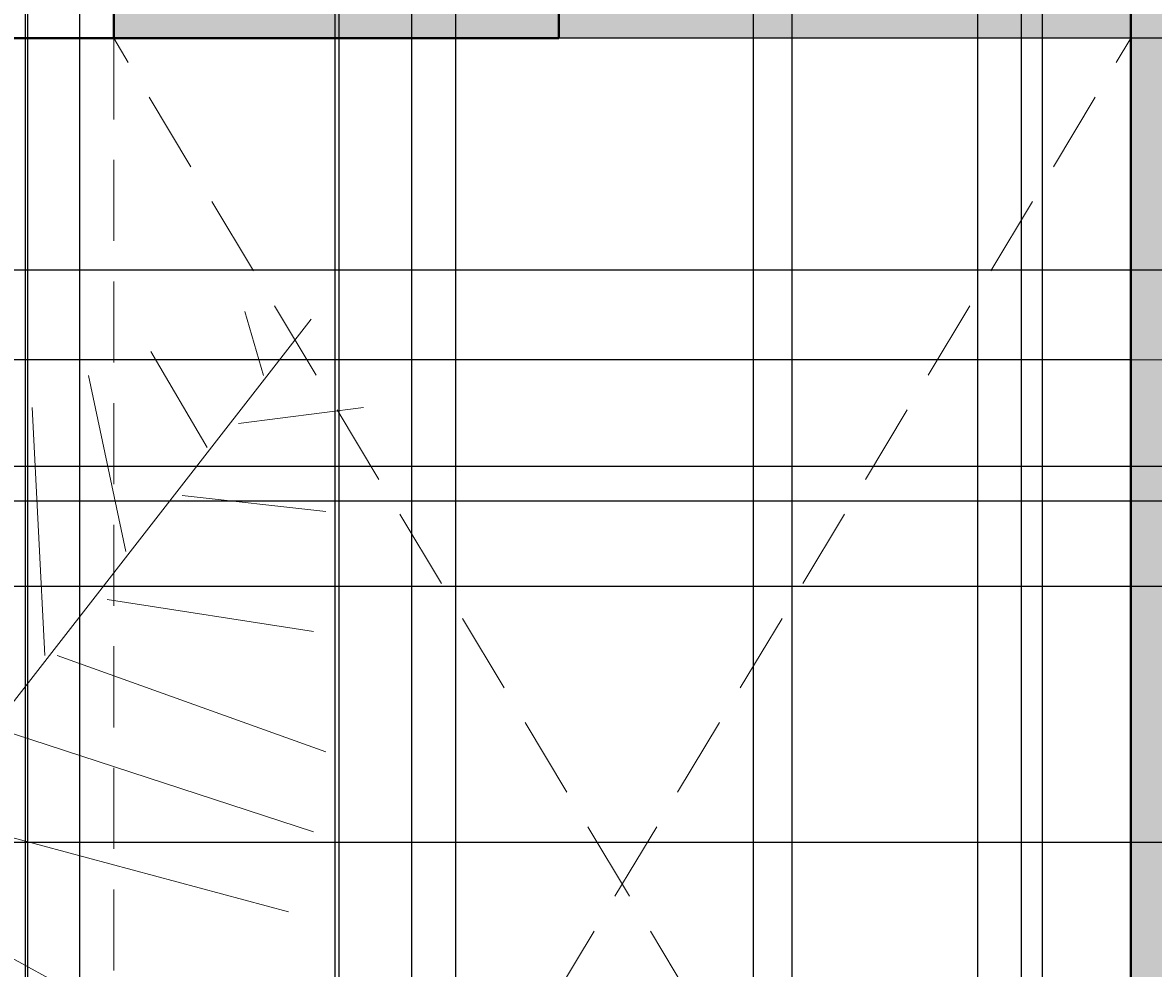
# Model space of a CAD drawing. Units: inches. Extents: x 818 to 1898, y 976 to 2364.
# Tile 65 of 96: x 1173 to 1260, y 1972 to 2045. Entities that reach past the tile are written whole.
import ezdxf

# ---------------------------------------------------------------- set-up
doc = ezdxf.new("R2010")
doc.units = ezdxf.units.IN
doc.header["$LTSCALE"] = 5
doc.header["$MEASUREMENT"] = 0
doc.linetypes.add('HIDDEN', pattern=[0.375, 0.25, -0.125])
for name, color, linetype, lineweight in [('A-ANNO-DIMS', 2, 'Continuous', 18), ('A-FLOR-OVHD', 8, 'HIDDEN', 13), ('A-GLAZ', 4, 'Continuous', 18), ('A-WALL', 7, 'Continuous', 40), ('A-WALL-HIDN', 7, 'HIDDEN', 18)]:
    doc.layers.add(name, color=color, linetype=linetype, lineweight=lineweight)
for name, color, linetype, lineweight, true_color in [('A-GLAZ-PATT', 141, 'Continuous', 9, 0xadddf7), ('A-WALL-PATT', 251, 'Continuous', 13, 0x636466), ('L-PLNT', 116, 'Continuous', 13, 0x136734)]:
    doc.layers.add(name, color=color, linetype=linetype, lineweight=lineweight, true_color=true_color)
doc.styles.get("Standard").update_dxf_attribs({"font": 'arial.ttf'})
doc.dimstyles.get("Standard").update_dxf_attribs({"dimtxt": 0.18, "dimasz": 0.18, "dimexe": 0.18, "dimexo": 0.0625, "dimgap": 0.09, "dimtad": 0, "dimtih": 1, "dimtoh": 1, "dimdec": 4, "dimzin": 0, "dimdsep": 46, "dimtxsty": 'Standard', "dimcen": 0.09, "dimadec": 0, "dimazin": 0, "dimtfac": 1, "dimtdec": 4, "dimtofl": 0, "dimtmove": 0, "dimatfit": 3, "dimfxl": 1, "dimtolj": 1, "dimtzin": 0, "dimarcsym": 0})

# ---------------------------------------------------------------- blocks, each defined once
blk = doc.blocks.new('PALM-DECK')
for p, q in [((132.87, 118.216), (134.313, 113.279)), ((110.075, 81.729), (137.983, 117.61)), ((125.649, 115.13), (129.981, 107.724)), ((120.834, 113.279), (123.723, 99.701)), ((116.502, 110.81), (117.465, 91.677)), ((132.389, 109.575), (142.017, 110.81)), ((128.056, 104.022), (139.128, 102.787)), ((122.279, 95.998), (138.165, 93.53)), ((118.427, 91.677), (139.128, 84.271)), ((113.613, 86.124), (138.165, 78.1)), ((106.393, 79.952), (136.239, 71.928)), ((98.208, 77.483), (120.834, 65.14))]:
    blk.add_line(p, q)
blk = doc.blocks.new('*D59')
at = {"layer": 'A-ANNO-DIMS', "color": 0, "lineweight": -2, "ltscale": 5, "transparency": 16777216}
for p, q in [((1251.643, 2300.393), (818.026, 2300.393)), ((818.206, 2300.213), (818.206, 1669.95)), ((818.206, 1039.323), (818.206, 1669.586)), ((896.051, 1039.143), (818.026, 1039.143))]:
    blk.add_line(p, q, dxfattribs=at)
at = {"layer": 'A-ANNO-DIMS', "color": 0, "ltscale": 5, "transparency": 16777216}
for points in [[(818.176, 2300.213), (818.236, 2300.213), (818.206, 2300.393)], [(818.176, 1039.323), (818.236, 1039.323), (818.206, 1039.143)]]:
    blk.add_solid(points, dxfattribs=at)
at = {"layer": 'Defpoints', "color": 0, "ltscale": 5, "transparency": 16777216}
for p in [(818.206, 2300.393), (1251.706, 2300.393), (896.114, 1039.143)]:
    blk.add_point(p, dxfattribs=at)
at = {"layer": 'A-ANNO-DIMS', "color": 0, "ltscale": 5, "transparency": 16777216, "insert": (818.206, 1669.768), "char_height": 0.18, "attachment_point": 5}
blk.add_mtext('\\A1;1261.2', dxfattribs=at)
blk = doc.blocks.new('*D61')
at = {"layer": 'A-ANNO-DIMS', "color": 0, "lineweight": -2, "ltscale": 5, "transparency": 16777216}
for p, q in [((1071.725, 1203.027), (1071.725, 2363.873)), ((1071.905, 2363.693), (1250.936, 2363.693)), ((1430.545, 2363.693), (1251.514, 2363.693)), ((1430.725, 1203.027), (1430.725, 2363.873))]:
    blk.add_line(p, q, dxfattribs=at)
at = {"layer": 'A-ANNO-DIMS', "color": 0, "ltscale": 5, "transparency": 16777216}
for points in [[(1071.905, 2363.723), (1071.905, 2363.663), (1071.725, 2363.693)], [(1430.545, 2363.723), (1430.545, 2363.663), (1430.725, 2363.693)]]:
    blk.add_solid(points, dxfattribs=at)
at = {"layer": 'Defpoints', "color": 0, "ltscale": 5, "transparency": 16777216}
for p in [(1430.725, 2363.693), (1071.725, 1202.964), (1430.725, 1202.964)]:
    blk.add_point(p, dxfattribs=at)
at = {"layer": 'A-ANNO-DIMS', "color": 0, "ltscale": 5, "transparency": 16777216, "insert": (1251.225, 2363.693), "char_height": 0.18, "attachment_point": 5}
blk.add_mtext('\\A1;359', dxfattribs=at)
blk = doc.blocks.new('*D64')
at = {"layer": 'A-ANNO-DIMS', "color": 0, "lineweight": -2, "ltscale": 5, "transparency": 16777216}
for p, q in [((1197.725, 1501.141), (1197.725, 2363.873)), ((1197.905, 2363.693), (1313.935, 2363.693)), ((1430.545, 2363.693), (1314.516, 2363.693)), ((1430.725, 1501.141), (1430.725, 2363.873))]:
    blk.add_line(p, q, dxfattribs=at)
at = {"layer": 'A-ANNO-DIMS', "color": 0, "ltscale": 5, "transparency": 16777216}
for points in [[(1197.905, 2363.723), (1197.905, 2363.663), (1197.725, 2363.693)], [(1430.545, 2363.723), (1430.545, 2363.663), (1430.725, 2363.693)]]:
    blk.add_solid(points, dxfattribs=at)
at = {"layer": 'Defpoints', "color": 0, "ltscale": 5, "transparency": 16777216}
for p in [(1430.725, 2363.693), (1197.725, 1501.078), (1430.725, 1501.078)]:
    blk.add_point(p, dxfattribs=at)
at = {"layer": 'A-ANNO-DIMS', "color": 0, "ltscale": 5, "transparency": 16777216, "insert": (1314.225, 2363.693), "char_height": 0.18, "attachment_point": 5}
blk.add_mtext('\\A1;233', dxfattribs=at)
blk = doc.blocks.new('*D73')
at = {"layer": 'A-ANNO-DIMS', "color": 0, "lineweight": -2, "ltscale": 5, "transparency": 16777216}
for p, q in [((1590.663, 2011.078), (818.026, 2011.078)), ((818.206, 2010.898), (818.206, 1996.76)), ((818.206, 1982.258), (818.206, 1996.396)), ((1590.663, 1982.078), (818.026, 1982.078))]:
    blk.add_line(p, q, dxfattribs=at)
at = {"layer": 'A-ANNO-DIMS', "color": 0, "ltscale": 5, "transparency": 16777216}
for points in [[(818.176, 2010.898), (818.236, 2010.898), (818.206, 2011.078)], [(818.176, 1982.258), (818.236, 1982.258), (818.206, 1982.078)]]:
    blk.add_solid(points, dxfattribs=at)
at = {"layer": 'Defpoints', "color": 0, "ltscale": 5, "transparency": 16777216}
for p in [(818.206, 2011.078), (1590.725, 2011.078), (1590.725, 1982.078)]:
    blk.add_point(p, dxfattribs=at)
at = {"layer": 'A-ANNO-DIMS', "color": 0, "ltscale": 5, "transparency": 16777216, "insert": (818.206, 1996.578), "char_height": 0.18, "attachment_point": 5}
blk.add_mtext('\\A1;29', dxfattribs=at)
blk = doc.blocks.new('*D82')
at = {"layer": 'A-ANNO-DIMS', "color": 0, "lineweight": -2, "ltscale": 5, "transparency": 16777216}
for p, q in [((1083.725, 1501.141), (1083.725, 2363.873)), ((1083.905, 2363.693), (1140.445, 2363.693)), ((1197.545, 2363.693), (1141.005, 2363.693)), ((1197.725, 1501.141), (1197.725, 2363.873))]:
    blk.add_line(p, q, dxfattribs=at)
at = {"layer": 'A-ANNO-DIMS', "color": 0, "ltscale": 5, "transparency": 16777216}
for points in [[(1083.905, 2363.723), (1083.905, 2363.663), (1083.725, 2363.693)], [(1197.545, 2363.723), (1197.545, 2363.663), (1197.725, 2363.693)]]:
    blk.add_solid(points, dxfattribs=at)
at = {"layer": 'Defpoints', "color": 0, "ltscale": 5, "transparency": 16777216}
for p in [(1197.725, 2363.693), (1083.725, 1501.078), (1197.725, 1501.078)]:
    blk.add_point(p, dxfattribs=at)
at = {"layer": 'A-ANNO-DIMS', "color": 0, "ltscale": 5, "transparency": 16777216, "insert": (1140.725, 2363.693), "char_height": 0.18, "attachment_point": 5}
blk.add_mtext('\\A1;114', dxfattribs=at)
blk = doc.blocks.new('*D83')
at = {"layer": 'A-ANNO-DIMS', "color": 0, "lineweight": -2, "ltscale": 5, "transparency": 16777216}
for p, q in [((1197.725, 1700.141), (1197.725, 2363.873)), ((1197.905, 2363.693), (1228.023, 2363.693)), ((1258.545, 2363.693), (1228.427, 2363.693)), ((1258.725, 1700.141), (1258.725, 2363.873))]:
    blk.add_line(p, q, dxfattribs=at)
at = {"layer": 'A-ANNO-DIMS', "color": 0, "ltscale": 5, "transparency": 16777216}
for points in [[(1197.905, 2363.723), (1197.905, 2363.663), (1197.725, 2363.693)], [(1258.545, 2363.723), (1258.545, 2363.663), (1258.725, 2363.693)]]:
    blk.add_solid(points, dxfattribs=at)
at = {"layer": 'Defpoints', "color": 0, "ltscale": 5, "transparency": 16777216}
for p in [(1258.725, 2363.693), (1197.725, 1700.078), (1258.725, 1700.078)]:
    blk.add_point(p, dxfattribs=at)
at = {"layer": 'A-ANNO-DIMS', "color": 0, "ltscale": 5, "transparency": 16777216, "insert": (1228.225, 2363.693), "char_height": 0.18, "attachment_point": 5}
blk.add_mtext('\\A1;61', dxfattribs=at)
blk = doc.blocks.new('*D85')
at = {"layer": 'A-ANNO-DIMS', "color": 0, "lineweight": -2, "ltscale": 5, "transparency": 16777216}
for p, q in [((1258.788, 2053.078), (1897.916, 2053.078)), ((1897.736, 2052.898), (1897.736, 1876.76)), ((1897.736, 1700.258), (1897.736, 1876.396)), ((1258.788, 1700.078), (1897.916, 1700.078))]:
    blk.add_line(p, q, dxfattribs=at)
at = {"layer": 'A-ANNO-DIMS', "color": 0, "ltscale": 5, "transparency": 16777216}
for points in [[(1897.706, 2052.898), (1897.766, 2052.898), (1897.736, 2053.078)], [(1897.706, 1700.258), (1897.766, 1700.258), (1897.736, 1700.078)]]:
    blk.add_solid(points, dxfattribs=at)
at = {"layer": 'Defpoints', "color": 0, "ltscale": 5, "transparency": 16777216}
for p in [(1258.725, 2053.078), (1897.736, 2053.078), (1258.725, 1700.078)]:
    blk.add_point(p, dxfattribs=at)
at = {"layer": 'A-ANNO-DIMS', "color": 0, "ltscale": 5, "transparency": 16777216, "insert": (1897.736, 1876.578), "char_height": 0.18, "attachment_point": 5}
blk.add_mtext('\\A1;353', dxfattribs=at)
blk = doc.blocks.new('*D94')
at = {"layer": 'A-ANNO-DIMS', "color": 0, "lineweight": -2, "ltscale": 5, "transparency": 16777216}
for p, q in [((1120.762, 1071.118), (1120.762, 2363.873)), ((1120.942, 2363.693), (1146.758, 2363.693)), ((1173.362, 2363.693), (1147.546, 2363.693)), ((1173.542, 1071.118), (1173.542, 2363.873))]:
    blk.add_line(p, q, dxfattribs=at)
at = {"layer": 'A-ANNO-DIMS', "color": 0, "ltscale": 5, "transparency": 16777216}
for points in [[(1120.942, 2363.723), (1120.942, 2363.663), (1120.762, 2363.693)], [(1173.362, 2363.723), (1173.362, 2363.663), (1173.542, 2363.693)]]:
    blk.add_solid(points, dxfattribs=at)
at = {"layer": 'Defpoints', "color": 0, "ltscale": 5, "transparency": 16777216}
for p in [(1173.542, 2363.693), (1120.762, 1071.055), (1173.542, 1071.055)]:
    blk.add_point(p, dxfattribs=at)
at = {"layer": 'A-ANNO-DIMS', "color": 0, "ltscale": 5, "transparency": 16777216, "insert": (1147.152, 2363.693), "char_height": 0.18, "attachment_point": 5}
blk.add_mtext('\\A1;52.78', dxfattribs=at)
blk = doc.blocks.new('*D95')
at = {"layer": 'A-ANNO-DIMS', "color": 0, "lineweight": -2, "ltscale": 5, "transparency": 16777216}
for p, q in [((1173.542, 1071.118), (1173.542, 2363.873)), ((1173.722, 2363.693), (1201.288, 2363.693)), ((1229.467, 2363.693), (1201.901, 2363.693)), ((1229.647, 1071.118), (1229.647, 2363.873))]:
    blk.add_line(p, q, dxfattribs=at)
at = {"layer": 'A-ANNO-DIMS', "color": 0, "ltscale": 5, "transparency": 16777216}
for points in [[(1173.722, 2363.723), (1173.722, 2363.663), (1173.542, 2363.693)], [(1229.467, 2363.723), (1229.467, 2363.663), (1229.647, 2363.693)]]:
    blk.add_solid(points, dxfattribs=at)
at = {"layer": 'Defpoints', "color": 0, "ltscale": 5, "transparency": 16777216}
for p in [(1229.647, 2363.693), (1173.542, 1071.055), (1229.647, 1071.055)]:
    blk.add_point(p, dxfattribs=at)
at = {"layer": 'A-ANNO-DIMS', "color": 0, "ltscale": 5, "transparency": 16777216, "insert": (1201.595, 2363.693), "char_height": 0.18, "attachment_point": 5}
blk.add_mtext('\\A1;56.1', dxfattribs=at)
blk = doc.blocks.new('*D96')
at = {"layer": 'A-ANNO-DIMS', "color": 0, "lineweight": -2, "ltscale": 5, "transparency": 16777216}
for p, q in [((1229.647, 1071.118), (1229.647, 2363.873)), ((1229.827, 2363.693), (1256.516, 2363.693)), ((1283.99, 2363.693), (1257.301, 2363.693)), ((1284.17, 1071.118), (1284.17, 2363.873))]:
    blk.add_line(p, q, dxfattribs=at)
at = {"layer": 'A-ANNO-DIMS', "color": 0, "ltscale": 5, "transparency": 16777216}
for points in [[(1229.827, 2363.723), (1229.827, 2363.663), (1229.647, 2363.693)], [(1283.99, 2363.723), (1283.99, 2363.663), (1284.17, 2363.693)]]:
    blk.add_solid(points, dxfattribs=at)
at = {"layer": 'Defpoints', "color": 0, "ltscale": 5, "transparency": 16777216}
for p in [(1284.17, 2363.693), (1229.647, 1071.055), (1284.17, 1071.055)]:
    blk.add_point(p, dxfattribs=at)
at = {"layer": 'A-ANNO-DIMS', "color": 0, "ltscale": 5, "transparency": 16777216, "insert": (1256.909, 2363.693), "char_height": 0.18, "attachment_point": 5}
blk.add_mtext('\\A1;54.52', dxfattribs=at)
blk = doc.blocks.new('*D109')
at = {"layer": 'A-ANNO-DIMS', "color": 0, "lineweight": -2, "ltscale": 5, "transparency": 16777216}
for p, q in [((1125.917, 1410.117), (1125.917, 2363.873)), ((1126.097, 2363.693), (1164.248, 2363.693)), ((1203.149, 2363.693), (1164.999, 2363.693)), ((1203.329, 1409.911), (1203.329, 2363.873))]:
    blk.add_line(p, q, dxfattribs=at)
at = {"layer": 'A-ANNO-DIMS', "color": 0, "ltscale": 5, "transparency": 16777216}
for points in [[(1126.097, 2363.723), (1126.097, 2363.663), (1125.917, 2363.693)], [(1203.149, 2363.723), (1203.149, 2363.663), (1203.329, 2363.693)]]:
    blk.add_solid(points, dxfattribs=at)
at = {"layer": 'Defpoints', "color": 0, "ltscale": 5, "transparency": 16777216}
for p in [(1203.329, 2363.693), (1125.917, 1410.055), (1203.329, 1409.848)]:
    blk.add_point(p, dxfattribs=at)
at = {"layer": 'A-ANNO-DIMS', "color": 0, "ltscale": 5, "transparency": 16777216, "insert": (1164.623, 2363.693), "char_height": 0.18, "attachment_point": 5}
blk.add_mtext('\\A1;77.41', dxfattribs=at)
blk = doc.blocks.new('*D145')
at = {"layer": 'A-ANNO-DIMS', "color": 0, "lineweight": -2, "ltscale": 5, "transparency": 16777216}
for p, q in [((1197.393, 2122.314), (1197.393, 975.663)), ((1232.609, 2122.314), (1232.609, 975.663)), ((1197.573, 975.843), (1214.608, 975.843)), ((1232.429, 975.843), (1215.394, 975.843))]:
    blk.add_line(p, q, dxfattribs=at)
at = {"layer": 'A-ANNO-DIMS', "color": 0, "ltscale": 5, "transparency": 16777216}
for points in [[(1197.573, 975.873), (1197.573, 975.813), (1197.393, 975.843)], [(1232.429, 975.873), (1232.429, 975.813), (1232.609, 975.843)]]:
    blk.add_solid(points, dxfattribs=at)
at = {"layer": 'Defpoints', "color": 0, "ltscale": 5, "transparency": 16777216}
for p in [(1197.393, 2122.377), (1232.609, 2122.377), (1232.609, 975.843)]:
    blk.add_point(p, dxfattribs=at)
at = {"layer": 'A-ANNO-DIMS', "color": 0, "ltscale": 5, "transparency": 16777216, "insert": (1215.001, 975.843), "char_height": 0.18, "attachment_point": 5}
blk.add_mtext('\\A1;35.22', dxfattribs=at)
blk = doc.blocks.new('*D158')
at = {"layer": 'A-ANNO-DIMS', "color": 0, "lineweight": -2, "ltscale": 5, "transparency": 16777216}
for p, q in [((1173.725, 1590.821), (1173.725, 2363.873)), ((1173.905, 2363.693), (1175.573, 2363.693)), ((1177.545, 2363.693), (1175.877, 2363.693)), ((1177.725, 1586.821), (1177.725, 2363.873))]:
    blk.add_line(p, q, dxfattribs=at)
at = {"layer": 'A-ANNO-DIMS', "color": 0, "ltscale": 5, "transparency": 16777216}
for points in [[(1173.905, 2363.723), (1173.905, 2363.663), (1173.725, 2363.693)], [(1177.545, 2363.723), (1177.545, 2363.663), (1177.725, 2363.693)]]:
    blk.add_solid(points, dxfattribs=at)
at = {"layer": 'Defpoints', "color": 0, "ltscale": 5, "transparency": 16777216}
for p in [(1177.725, 2363.693), (1173.725, 1590.758), (1177.725, 1586.758)]:
    blk.add_point(p, dxfattribs=at)
at = {"layer": 'A-ANNO-DIMS', "color": 0, "ltscale": 5, "transparency": 16777216, "insert": (1175.725, 2363.693), "char_height": 0.18, "attachment_point": 5}
blk.add_mtext('\\A1;4', dxfattribs=at)
blk = doc.blocks.new('*D207')
at = {"layer": 'A-ANNO-DIMS', "color": 0, "lineweight": -2, "ltscale": 5, "transparency": 16777216}
for p, q in [((1590.663, 2044.078), (818.026, 2044.078)), ((818.206, 2043.898), (818.206, 2027.76)), ((818.206, 2011.258), (818.206, 2027.396)), ((1590.663, 2011.078), (818.026, 2011.078))]:
    blk.add_line(p, q, dxfattribs=at)
at = {"layer": 'A-ANNO-DIMS', "color": 0, "ltscale": 5, "transparency": 16777216}
for points in [[(818.176, 2043.898), (818.236, 2043.898), (818.206, 2044.078)], [(818.176, 2011.258), (818.236, 2011.258), (818.206, 2011.078)]]:
    blk.add_solid(points, dxfattribs=at)
at = {"layer": 'Defpoints', "color": 0, "ltscale": 5, "transparency": 16777216}
for p in [(818.206, 2044.078), (1590.725, 2044.078), (1590.725, 2011.078)]:
    blk.add_point(p, dxfattribs=at)
at = {"layer": 'A-ANNO-DIMS', "color": 0, "ltscale": 5, "transparency": 16777216, "insert": (818.206, 2027.578), "char_height": 0.18, "attachment_point": 5}
blk.add_mtext('\\A1;33', dxfattribs=at)
blk = doc.blocks.new('*D232')
at = {"layer": 'A-ANNO-DIMS', "color": 0, "lineweight": -2, "ltscale": 5, "transparency": 16777216}
for p, q in [((1303.869, 2008.392), (818.026, 2008.392)), ((818.206, 2008.212), (818.206, 1980.898)), ((818.206, 1953.221), (818.206, 1980.534)), ((1303.869, 1953.041), (818.026, 1953.041))]:
    blk.add_line(p, q, dxfattribs=at)
at = {"layer": 'A-ANNO-DIMS', "color": 0, "ltscale": 5, "transparency": 16777216}
for points in [[(818.176, 2008.212), (818.236, 2008.212), (818.206, 2008.392)], [(818.176, 1953.221), (818.236, 1953.221), (818.206, 1953.041)]]:
    blk.add_solid(points, dxfattribs=at)
at = {"layer": 'Defpoints', "color": 0, "ltscale": 5, "transparency": 16777216}
for p in [(818.206, 2008.392), (1303.931, 2008.392), (1303.931, 1953.041)]:
    blk.add_point(p, dxfattribs=at)
at = {"layer": 'A-ANNO-DIMS', "color": 0, "ltscale": 5, "transparency": 16777216, "insert": (818.206, 1980.716), "char_height": 0.18, "attachment_point": 5}
blk.add_mtext('\\A1;55.35', dxfattribs=at)
blk = doc.blocks.new('*D234')
at = {"layer": 'A-ANNO-DIMS', "color": 0, "lineweight": -2, "ltscale": 5, "transparency": 16777216}
for p, q in [((1267.663, 2044.078), (818.026, 2044.078)), ((818.206, 2043.898), (818.206, 2026.417)), ((818.206, 2008.572), (818.206, 2026.053)), ((1303.869, 2008.392), (818.026, 2008.392))]:
    blk.add_line(p, q, dxfattribs=at)
at = {"layer": 'A-ANNO-DIMS', "color": 0, "ltscale": 5, "transparency": 16777216}
for points in [[(818.176, 2043.898), (818.236, 2043.898), (818.206, 2044.078)], [(818.176, 2008.572), (818.236, 2008.572), (818.206, 2008.392)]]:
    blk.add_solid(points, dxfattribs=at)
at = {"layer": 'Defpoints', "color": 0, "ltscale": 5, "transparency": 16777216}
for p in [(818.206, 2044.078), (1267.725, 2044.078), (1303.931, 2008.392)]:
    blk.add_point(p, dxfattribs=at)
at = {"layer": 'A-ANNO-DIMS', "color": 0, "ltscale": 5, "transparency": 16777216, "insert": (818.206, 2026.235), "char_height": 0.18, "attachment_point": 5}
blk.add_mtext('\\A1;35.69', dxfattribs=at)
blk = doc.blocks.new('*D237')
at = {"layer": 'A-ANNO-DIMS', "color": 0, "lineweight": -2, "ltscale": 5, "transparency": 16777216}
for p, q in [((1310.845, 2026.207), (818.026, 2026.207)), ((818.206, 2026.027), (818.206, 2014.198)), ((818.206, 2002.005), (818.206, 2013.834)), ((1314.197, 2001.825), (818.026, 2001.825))]:
    blk.add_line(p, q, dxfattribs=at)
at = {"layer": 'A-ANNO-DIMS', "color": 0, "ltscale": 5, "transparency": 16777216}
for points in [[(818.176, 2026.027), (818.236, 2026.027), (818.206, 2026.207)], [(818.176, 2002.005), (818.236, 2002.005), (818.206, 2001.825)]]:
    blk.add_solid(points, dxfattribs=at)
at = {"layer": 'Defpoints', "color": 0, "ltscale": 5, "transparency": 16777216}
for p in [(1310.908, 2026.207), (818.206, 2001.825), (1314.26, 2001.825)]:
    blk.add_point(p, dxfattribs=at)
at = {"layer": 'A-ANNO-DIMS', "color": 0, "ltscale": 5, "transparency": 16777216, "insert": (818.206, 2014.016), "char_height": 0.18, "attachment_point": 5}
blk.add_mtext('\\A1;24.383', dxfattribs=at)
blk = doc.blocks.new('*D248')
at = {"layer": 'A-ANNO-DIMS', "color": 0, "lineweight": -2, "ltscale": 5, "transparency": 16777216}
for p, q in [((1258.663, 2019.287), (818.026, 2019.287)), ((818.206, 2019.107), (818.206, 1974.286)), ((818.206, 1929.102), (818.206, 1973.922)), ((1258.663, 1928.922), (818.026, 1928.922))]:
    blk.add_line(p, q, dxfattribs=at)
at = {"layer": 'A-ANNO-DIMS', "color": 0, "ltscale": 5, "transparency": 16777216}
for points in [[(818.176, 2019.107), (818.236, 2019.107), (818.206, 2019.287)], [(818.176, 1929.102), (818.236, 1929.102), (818.206, 1928.922)]]:
    blk.add_solid(points, dxfattribs=at)
at = {"layer": 'Defpoints', "color": 0, "ltscale": 5, "transparency": 16777216}
for p in [(818.206, 2019.287), (1258.725, 2019.287), (1258.725, 1928.922)]:
    blk.add_point(p, dxfattribs=at)
at = {"layer": 'A-ANNO-DIMS', "color": 0, "ltscale": 5, "transparency": 16777216, "insert": (818.206, 1974.104), "char_height": 0.18, "attachment_point": 5}
blk.add_mtext('\\A1;90.37', dxfattribs=at)
blk = doc.blocks.new('*D269')
at = {"layer": 'A-ANNO-DIMS', "color": 0, "lineweight": -2, "ltscale": 5, "transparency": 16777216}
for p, q in [((1246.938, 1534.141), (1246.938, 2363.873)), ((1247.118, 2363.693), (1293.706, 2363.693)), ((1341.079, 2363.693), (1294.491, 2363.693)), ((1341.259, 1534.141), (1341.259, 2363.873))]:
    blk.add_line(p, q, dxfattribs=at)
at = {"layer": 'A-ANNO-DIMS', "color": 0, "ltscale": 5, "transparency": 16777216}
for points in [[(1247.118, 2363.723), (1247.118, 2363.663), (1246.938, 2363.693)], [(1341.079, 2363.723), (1341.079, 2363.663), (1341.259, 2363.693)]]:
    blk.add_solid(points, dxfattribs=at)
at = {"layer": 'Defpoints', "color": 0, "ltscale": 5, "transparency": 16777216}
for p in [(1341.259, 2363.693), (1246.938, 1534.078), (1341.259, 1534.078)]:
    blk.add_point(p, dxfattribs=at)
at = {"layer": 'A-ANNO-DIMS', "color": 0, "ltscale": 5, "transparency": 16777216, "insert": (1294.099, 2363.693), "char_height": 0.18, "attachment_point": 5}
blk.add_mtext('\\A1;94.32', dxfattribs=at)
blk = doc.blocks.new('*D271')
at = {"layer": 'A-ANNO-DIMS', "color": 0, "lineweight": -2, "ltscale": 5, "transparency": 16777216}
for p, q in [((1206.725, 1510.141), (1206.725, 2363.873)), ((1206.905, 2363.693), (1226.451, 2363.693)), ((1246.758, 2363.693), (1227.211, 2363.693)), ((1246.938, 1510.141), (1246.938, 2363.873))]:
    blk.add_line(p, q, dxfattribs=at)
at = {"layer": 'A-ANNO-DIMS', "color": 0, "ltscale": 5, "transparency": 16777216}
for points in [[(1206.905, 2363.723), (1206.905, 2363.663), (1206.725, 2363.693)], [(1246.758, 2363.723), (1246.758, 2363.663), (1246.938, 2363.693)]]:
    blk.add_solid(points, dxfattribs=at)
at = {"layer": 'Defpoints', "color": 0, "ltscale": 5, "transparency": 16777216}
for p in [(1246.938, 2363.693), (1206.725, 1510.078), (1246.938, 1510.078)]:
    blk.add_point(p, dxfattribs=at)
at = {"layer": 'A-ANNO-DIMS', "color": 0, "ltscale": 5, "transparency": 16777216, "insert": (1226.831, 2363.693), "char_height": 0.18, "attachment_point": 5}
blk.add_mtext('\\A1;40.21', dxfattribs=at)
blk = doc.blocks.new('*D276')
at = {"layer": 'A-ANNO-DIMS', "color": 0, "lineweight": -2, "ltscale": 5, "transparency": 16777216}
for p, q in [((1206.725, 1687.141), (1206.725, 2363.873)), ((1206.905, 2363.693), (1228.949, 2363.693)), ((1251.753, 2363.693), (1229.709, 2363.693)), ((1251.933, 1681.439), (1251.933, 2363.873))]:
    blk.add_line(p, q, dxfattribs=at)
at = {"layer": 'A-ANNO-DIMS', "color": 0, "ltscale": 5, "transparency": 16777216}
for points in [[(1206.905, 2363.723), (1206.905, 2363.663), (1206.725, 2363.693)], [(1251.753, 2363.723), (1251.753, 2363.663), (1251.933, 2363.693)]]:
    blk.add_solid(points, dxfattribs=at)
at = {"layer": 'Defpoints', "color": 0, "ltscale": 5, "transparency": 16777216}
for p in [(1251.933, 2363.693), (1206.725, 1687.078), (1251.933, 1681.376)]:
    blk.add_point(p, dxfattribs=at)
at = {"layer": 'A-ANNO-DIMS', "color": 0, "ltscale": 5, "transparency": 16777216, "insert": (1229.329, 2363.693), "char_height": 0.18, "attachment_point": 5}
blk.add_mtext('\\A1;45.21', dxfattribs=at)
blk = doc.blocks.new('*D281')
at = {"layer": 'A-ANNO-DIMS', "color": 0, "lineweight": -2, "ltscale": 5, "transparency": 16777216}
for p, q in [((1250.303, 1913.703), (1250.303, 2363.873)), ((1250.483, 2363.693), (1420.121, 2363.693)), ((1590.545, 2363.693), (1420.907, 2363.693)), ((1590.725, 2011.141), (1590.725, 2363.873))]:
    blk.add_line(p, q, dxfattribs=at)
at = {"layer": 'A-ANNO-DIMS', "color": 0, "ltscale": 5, "transparency": 16777216}
for points in [[(1250.483, 2363.723), (1250.483, 2363.663), (1250.303, 2363.693)], [(1590.545, 2363.723), (1590.545, 2363.663), (1590.725, 2363.693)]]:
    blk.add_solid(points, dxfattribs=at)
at = {"layer": 'Defpoints', "color": 0, "ltscale": 5, "transparency": 16777216}
for p in [(1590.725, 2363.693), (1590.725, 2011.078), (1250.303, 1913.64)]:
    blk.add_point(p, dxfattribs=at)
at = {"layer": 'A-ANNO-DIMS', "color": 0, "ltscale": 5, "transparency": 16777216, "insert": (1420.514, 2363.693), "char_height": 0.18, "attachment_point": 5}
blk.add_mtext('\\A1;340.4', dxfattribs=at)

msp = doc.modelspace()

# ---------------------------------------------------------------- hatches: boundary and pattern name
at = {"layer": 'A-GLAZ-PATT', "ltscale": 5}
h = msp.add_hatch(color=256, dxfattribs=at)
h.dxf.hatch_style = 1
h.paths.add_polyline_path([(1283.8183, 1504.5782), (1206.7251, 1504.5782), (1206.7251, 1501.0782), (1283.8183, 1501.0782)])
h.paths.add_polyline_path([(1283.8183, 1510.0782), (1206.7251, 1510.0782), (1206.7251, 1506.5782), (1283.8183, 1506.5782)])
h.paths.add_polyline_path([(1490.9163, 1355.0782), (1439.7252, 1355.0782), (1439.7252, 1409.0522), (1436.2252, 1409.0522), (1436.2252, 1351.5782), (1490.9163, 1351.5782)])
h.paths.add_polyline_path([(1434.2252, 1409.0522), (1430.7251, 1409.0522), (1430.7251, 1346.0782), (1435.0799, 1346.0782), (1435.0731, 1346.1152), (1435.1501, 1346.0782), (1490.9163, 1346.0782), (1490.9163, 1349.5782), (1434.2252, 1349.5782)])
h.paths.add_polyline_path([(1714.7252, 1545.0782), (1711.2252, 1545.0782), (1711.2252, 1521.0782), (1714.7252, 1521.0782)])
h.paths.add_polyline_path([(1709.2252, 1545.0782), (1705.7252, 1545.0782), (1705.7252, 1521.0782), (1709.2252, 1521.0782)])
h.paths.add_polyline_path([(1714.7252, 1687.0782), (1711.2252, 1687.0782), (1711.2252, 1649.9029), (1714.7252, 1649.9029)])
h.paths.add_polyline_path([(1709.2252, 1687.0782), (1705.7252, 1687.0782), (1705.7252, 1649.9029), (1709.2252, 1649.9029)])
h.paths.add_polyline_path([(1709.2252, 1745.5584), (1705.7252, 1745.5584), (1705.7252, 1717.3178), (1709.2252, 1717.3178)])
h.paths.add_polyline_path([(1714.7252, 1745.5584), (1711.2252, 1745.5584), (1711.2252, 1717.3178), (1714.7252, 1717.3178)])
h.paths.add_polyline_path([(1714.7252, 2014.5114), (1711.2252, 2014.5114), (1711.2252, 1962.0338), (1714.7252, 1962.0338)])
h.paths.add_polyline_path([(1709.2252, 2014.5114), (1705.7252, 2014.5114), (1705.7252, 1962.0338), (1709.2252, 1962.0338)])
h.paths.add_polyline_path([(1538.5155, 2047.5782), (1485.1216, 2047.5782), (1485.1216, 2044.0782), (1538.5155, 2044.0782)])
h.paths.add_polyline_path([(1538.5155, 2053.0782), (1485.1216, 2053.0782), (1485.1216, 2049.5782), (1538.5155, 2049.5782)])
h.paths.add_polyline_path([(1388.0315, 2047.5782), (1330.305, 2047.5782), (1330.305, 2044.0782), (1388.0315, 2044.0782)])
h.paths.add_polyline_path([(1388.0315, 2053.0782), (1330.305, 2053.0782), (1330.305, 2049.5782), (1388.0315, 2049.5782)])
h.paths.add_polyline_path([(1262.2252, 2019.2871), (1258.7251, 2019.2871), (1258.7251, 1928.9218), (1262.2252, 1928.9218)])
h.paths.add_polyline_path([(1267.7251, 2019.2871), (1264.2252, 2019.2871), (1264.2252, 1928.9218), (1267.7251, 1928.9218)])
h.paths.add_polyline_path([(1262.2252, 1862.9652), (1258.7251, 1862.9652), (1258.7251, 1814.9652), (1262.2252, 1814.9652)])
h.paths.add_polyline_path([(1267.7251, 1862.9652), (1264.2252, 1862.9652), (1264.2252, 1814.9652), (1267.7251, 1814.9652)])
h.paths.add_polyline_path([(1262.2252, 1755.3321), (1258.7251, 1755.3321), (1258.7251, 1707.3321), (1262.2252, 1707.3321)])
h.paths.add_polyline_path([(1267.7251, 1755.3321), (1264.2252, 1755.3321), (1264.2252, 1707.3321), (1267.7251, 1707.3321)])
h.paths.add_polyline_path([(1251.9333, 1692.5782), (1206.7251, 1692.5782), (1206.7251, 1687.0782), (1251.9333, 1687.0782)])
h.paths.add_polyline_path([(1251.9333, 1700.0782), (1206.7251, 1700.0782), (1206.7251, 1694.5782), (1251.9333, 1694.5782)])
at = {"layer": 'A-WALL-PATT', "ltscale": 5}
h = msp.add_hatch(color=256, dxfattribs=at)
h.dxf.hatch_style = 1
h.paths.add_polyline_path([(1267.7251, 1928.9218), (1258.7251, 1928.9218), (1258.7251, 1913.6401), (1250.3029, 1913.6401), (1250.3029, 1878.3919), (1258.7251, 1878.3919), (1258.7251, 1862.9652), (1267.7251, 1862.9652)])
h.paths.add_polyline_path([(1267.7251, 1814.9652), (1258.7251, 1814.9652), (1258.7251, 1755.3321), (1267.7251, 1755.3321)])
h.paths.add_polyline_path([(1463.7252, 1696.0782), (1267.7251, 1696.0782), (1267.7251, 1707.3321), (1258.7251, 1707.3321), (1258.7251, 1700.0782), (1251.9333, 1700.0782), (1251.9333, 1687.0782), (1463.7252, 1687.0782)])
h.paths.add_polyline_path([(1714.7252, 1717.3178), (1705.7252, 1717.3178), (1705.7252, 1696.0782), (1599.7252, 1696.0782), (1599.7252, 1790.0782), (1705.7252, 1790.0782), (1705.7252, 1785.6125), (1714.7252, 1785.6125), (1714.7252, 1827.2125), (1705.7252, 1827.2125), (1705.7252, 1802.0782), (1599.7252, 1802.0782), (1599.7252, 1867.0782), (1705.7252, 1867.0782), (1705.7252, 1857.2125), (1714.7252, 1857.2125), (1714.7252, 1930.0316), (1741.8409, 1930.0316), (1741.8409, 1935.0316), (1714.7252, 1935.0316), (1714.7252, 1957.0338), (1741.8409, 1957.0338), (1741.8409, 1962.0338), (1714.7252, 1962.0338), (1705.7252, 1962.0338), (1705.7252, 1948.0782), (1599.7252, 1948.0782), (1599.7252, 1981.0782), (1590.7251, 1981.0782), (1590.7251, 1941.0782), (1620.7252, 1941.0782), (1705.7252, 1941.0782), (1705.7252, 1876.0782), (1599.7252, 1876.0782), (1599.7252, 1911.0782), (1590.7251, 1911.0782), (1590.7251, 1876.0782), (1429.2252, 1876.0782), (1429.2252, 1867.0782), (1511.7252, 1867.0782), (1528.593, 1867.0782), (1595.7252, 1867.0782), (1595.7252, 1773.0782), (1520.7252, 1773.0782), (1520.7252, 1837.5823), (1532.593, 1837.5823), (1532.593, 1867.0782), (1528.593, 1867.0782), (1528.593, 1841.5823), (1511.7252, 1841.5823), (1511.7252, 1744.9714), (1520.7252, 1744.9714), (1520.7252, 1761.0782), (1595.7252, 1761.0782), (1595.7252, 1696.0782), (1520.7252, 1696.0782), (1520.7252, 1716.0454), (1511.7252, 1716.0454), (1511.7252, 1696.0782), (1511.7252, 1687.0782), (1714.7252, 1687.0782)])
h.paths.add_polyline_path([(1714.7252, 2053.0782), (1714.7252, 2081.1881), (1709.7252, 2081.1881), (1709.7252, 2053.0782), (1681.6446, 2053.0782), (1681.6446, 2081.1881), (1676.6446, 2081.1881), (1676.6446, 2053.0782), (1538.5155, 2053.0782), (1538.5155, 2044.0782), (1590.7251, 2044.0782), (1590.7251, 2011.0782), (1599.7252, 2011.0782), (1599.7252, 2044.0782), (1705.7252, 2044.0782), (1705.7252, 2014.5114), (1714.7252, 2014.5114)])
h.paths.add_polyline_path([(1485.1216, 2053.0782), (1422.02, 2053.0782), (1422.02, 2081.1881), (1413.02, 2081.1881), (1413.02, 2053.0782), (1399.6356, 2053.0782), (1399.6356, 2081.1881), (1390.6356, 2081.1881), (1390.6356, 2053.0782), (1388.0315, 2053.0782), (1388.0315, 2044.0782), (1416.2743, 2044.0782), (1485.1216, 2044.0782)])
h.paths.add_polyline_path([(1330.305, 2053.0782), (1258.7251, 2053.0782), (1258.7251, 2019.2871), (1267.7251, 2019.2871), (1267.7251, 2044.0782), (1330.305, 2044.0782)])
h.paths.add_polyline_path([(1258.7251, 2053.0782), (1214.6577, 2053.0782), (1214.6577, 2044.0782), (1258.7251, 2044.0782)])
h.paths.add_polyline_path([(1214.6577, 2053.0782), (1180.349, 2053.0782), (1180.349, 2044.0782), (1214.6577, 2044.0782)])
h.paths.add_polyline_path([(1714.7252, 1639.5782), (1741.8409, 1639.5782), (1741.8409, 1643.5782), (1714.7252, 1643.5782), (1714.7252, 1649.9029), (1705.7252, 1649.9029), (1705.7252, 1600.0782), (1477.7252, 1600.0782), (1477.7252, 1591.0782), (1520.7252, 1591.0782), (1616.7252, 1591.0782), (1616.7252, 1416.6857), (1622.7252, 1416.6857), (1622.7252, 1463.0782), (1624.7252, 1463.0782), (1624.7252, 1467.0782), (1622.7252, 1467.0782), (1622.7252, 1591.0782), (1705.7252, 1591.0782), (1705.7252, 1545.0782), (1714.7252, 1545.0782), (1741.8409, 1545.0782), (1741.8409, 1549.0782), (1714.7252, 1549.0782), (1714.7252, 1593.9175), (1737.8409, 1593.9175), (1737.8409, 1597.9175), (1714.7252, 1597.9175)])
h.paths.add_polyline_path([(1674.9024, 2060.7419), (1714.7045, 2060.7419), (1714.7045, 2073.1061), (1674.9024, 2073.1061)], flags=25)
h.paths.add_polyline_path([(1394.5468, 2061.6618), (1422.2344, 2061.6618), (1422.2344, 2074.0261), (1394.5468, 2074.0261)], flags=24)

# ---------------------------------------------------------------- linework, layer by layer
at = {"layer": 'A-FLOR-OVHD', "ltscale": 5}
for p, q in [((1258.7251, 1913.6401), (1180.349, 2044.0782)), ((1180.349, 2044.0782), (1180.349, 1913.6401)), ((1180.349, 1913.6401), (1258.7251, 2044.0782))]:
    msp.add_line(p, q, dxfattribs=at)
at = {"layer": 'A-GLAZ'}
msp.add_line((1267.7251, 2019.2871), (1258.7251, 2019.2871), dxfattribs=at)
at = {"layer": 'A-WALL', "ltscale": 5}
for p, q in [((1180.349, 2053.0782), (1180.349, 2044.0782)), ((1214.6577, 2053.0782), (1214.6577, 2044.0782))]:
    msp.add_line(p, q, dxfattribs=at)
at = {"layer": 'A-WALL'}
for p, q in [((1258.7251, 2053.0782), (1258.7251, 1913.6401)), ((1083.7251, 2044.0782), (1214.6577, 2044.0782))]:
    msp.add_line(p, q, dxfattribs=at)
at = {"layer": 'A-WALL-HIDN', "ltscale": 5}
msp.add_line((1214.6577, 2044.0782), (1258.7251, 2044.0782), dxfattribs=at)

# ---------------------------------------------------------------- block references
at = {"layer": 'L-PLNT'}
msp.add_blockref('PALM-DECK', (1057.571, 1904.8049), dxfattribs=at)

# ---------------------------------------------------------------- dimensions: what is measured, and where the dimension line sits
at = {"layer": 'A-ANNO-DIMS', "ltscale": 5}
for base, p1, p2, override, picture, middle in [((1430.7251, 2363.6929), (1071.7251, 1202.9642), (1430.7251, 1202.9642), {"dimdec": 0, "dimlfac": 1, "dimrnd": 0, "dimzin": 0, "dimdsep": 46, "dimlunit": 2}, '*D61', (1251.2251, 2363.6929)), ((1197.7251, 2363.6929), (1083.7251, 1501.0782), (1197.7251, 1501.0782), {"dimdec": 0, "dimlfac": 1, "dimrnd": 0, "dimzin": 0, "dimdsep": 46, "dimlunit": 2}, '*D82', (1140.7251, 2363.6929)), ((1173.5418, 2363.6929), (1120.7618, 1071.0552), (1173.5418, 1071.0552), {"dimdec": 2, "dimlfac": 1, "dimrnd": 0, "dimzin": 0, "dimdsep": 46, "dimlunit": 2}, '*D94', (1147.1518, 2363.6929)), ((1203.3292, 2363.6929), (1125.9172, 1410.0547), (1203.3292, 1409.8484), {"dimdec": 2, "dimlfac": 1, "dimrnd": 0, "dimzin": 0, "dimdsep": 46, "dimlunit": 2}, '*D109', (1164.6232, 2363.6929)), ((1229.6474, 2363.6929), (1173.5418, 1071.0552), (1229.6474, 1071.0552), {"dimdec": 1, "dimlfac": 1, "dimrnd": 0, "dimzin": 0, "dimdsep": 46, "dimlunit": 2}, '*D95', (1201.5946, 2363.6929)), ((1177.7251, 2363.6929), (1173.7251, 1590.7585), (1177.7251, 1586.7585), {"dimdec": 0, "dimlfac": 1, "dimrnd": 0, "dimzin": 0, "dimdsep": 46, "dimlunit": 2}, '*D158', (1175.7251, 2363.6929)), ((1430.7251, 2363.6929), (1197.7251, 1501.0782), (1430.7251, 1501.0782), {"dimdec": 0, "dimlfac": 1, "dimrnd": 0, "dimzin": 0, "dimdsep": 46, "dimlunit": 2}, '*D64', (1314.2251, 2363.6929)), ((1258.7251, 2363.6929), (1197.7251, 1700.0782), (1258.7251, 1700.0782), {"dimdec": 0, "dimlfac": 1, "dimrnd": 0, "dimzin": 0, "dimdsep": 46, "dimlunit": 2}, '*D83', (1228.2251, 2363.6929)), ((1246.9377, 2363.6929), (1206.7251, 1510.0782), (1246.9377, 1510.0782), {"dimdec": 2, "dimlfac": 1, "dimrnd": 0, "dimzin": 0, "dimdsep": 46, "dimlunit": 2}, '*D271', (1226.8314, 2363.6929)), ((1251.9333, 2363.6929), (1206.7251, 1687.0782), (1251.9333, 1681.3763), {"dimdec": 2, "dimlfac": 1, "dimrnd": 0, "dimzin": 0, "dimdsep": 46, "dimlunit": 2}, '*D276', (1229.3292, 2363.6929)), ((1284.1697, 2363.6929), (1229.6474, 1071.0552), (1284.1697, 1071.0552), {"dimdec": 2, "dimlfac": 1, "dimrnd": 0, "dimzin": 0, "dimdsep": 46, "dimlunit": 2}, '*D96', (1256.9085, 2363.6929)), ((1341.2593, 2363.6929), (1246.9377, 1534.0782), (1341.2593, 1534.0782), {"dimdec": 2, "dimlfac": 1, "dimrnd": 0, "dimzin": 0, "dimdsep": 46, "dimlunit": 2}, '*D269', (1294.0985, 2363.6929)), ((1590.7251, 2363.6929), (1250.3029, 1913.6401), (1590.7251, 2011.0782), {"dimdec": 1, "dimlfac": 1, "dimrnd": 0, "dimzin": 0, "dimdsep": 46, "dimlunit": 2}, '*D281', (1420.514, 2363.6929)), ((1232.6091, 975.8433), (1197.3925, 2122.3767), (1232.6091, 2122.3767), {"dimdec": 2, "dimlfac": 1, "dimrnd": 0, "dimzin": 0, "dimdsep": 46, "dimlunit": 2}, '*D145', (1215.0008, 975.8433))]:
    dim = msp.add_linear_dim(base=base, p1=p1, p2=p2, dimstyle='Standard', override=override, dxfattribs=at)
    dim.commit()
    dim.dimension.update_dxf_attribs({"geometry": picture, "text_midpoint": middle})
for base, p1, p2, override, picture, middle in [((818.2059, 2300.3929), (896.1138, 1039.1433), (1251.7057, 2300.3929), {"dimdec": 1, "dimlfac": 1, "dimrnd": 0, "dimzin": 0, "dimdsep": 46, "dimlunit": 2}, '*D59', (818.2059, 1669.7681)), ((1897.736, 2053.0782), (1258.7251, 1700.0782), (1258.7251, 2053.0782), {"dimdec": 0, "dimlfac": 1, "dimrnd": 0, "dimzin": 0, "dimdsep": 46, "dimlunit": 2}, '*D85', (1897.736, 1876.5782)), ((818.2059, 2044.0782), (1303.9314, 2008.3917), (1267.7251, 2044.0782), {"dimdec": 2, "dimlfac": 1, "dimrnd": 0, "dimzin": 0, "dimdsep": 46, "dimlunit": 2}, '*D234', (818.2059, 2026.235)), ((818.2059, 2044.0782), (1590.7251, 2011.0782), (1590.7251, 2044.0782), {"dimdec": 0, "dimlfac": 1, "dimrnd": 0, "dimzin": 0, "dimdsep": 46, "dimlunit": 2}, '*D207', (818.2059, 2027.5782)), ((818.2059, 2001.8247), (1310.9077, 2026.2074), (1314.2595, 2001.8247), {"dimdec": 3, "dimlfac": 1, "dimrnd": 0, "dimzin": 0, "dimdsep": 46, "dimlunit": 2}, '*D237', (818.2059, 2014.016)), ((818.2059, 2019.2871), (1258.7251, 1928.9218), (1258.7251, 2019.2871), {"dimdec": 2, "dimlfac": 1, "dimrnd": 0, "dimzin": 0, "dimdsep": 46, "dimlunit": 2}, '*D248', (818.2059, 1974.1044)), ((818.2059, 2011.0782), (1590.7251, 1982.0782), (1590.7251, 2011.0782), {"dimdec": 0, "dimlfac": 1, "dimrnd": 0, "dimzin": 0, "dimdsep": 46, "dimlunit": 2}, '*D73', (818.2059, 1996.5782)), ((818.2059, 2008.3917), (1303.9314, 1953.0408), (1303.9314, 2008.3917), {"dimdec": 2, "dimlfac": 1, "dimrnd": 0, "dimzin": 0, "dimdsep": 46, "dimlunit": 2}, '*D232', (818.2059, 1980.7163))]:
    dim = msp.add_linear_dim(base=base, p1=p1, p2=p2, angle=90, dimstyle='Standard', override=override, dxfattribs=at)
    dim.commit()
    dim.dimension.update_dxf_attribs({"geometry": picture, "text_midpoint": middle})

doc.saveas('drawing.dxf')
